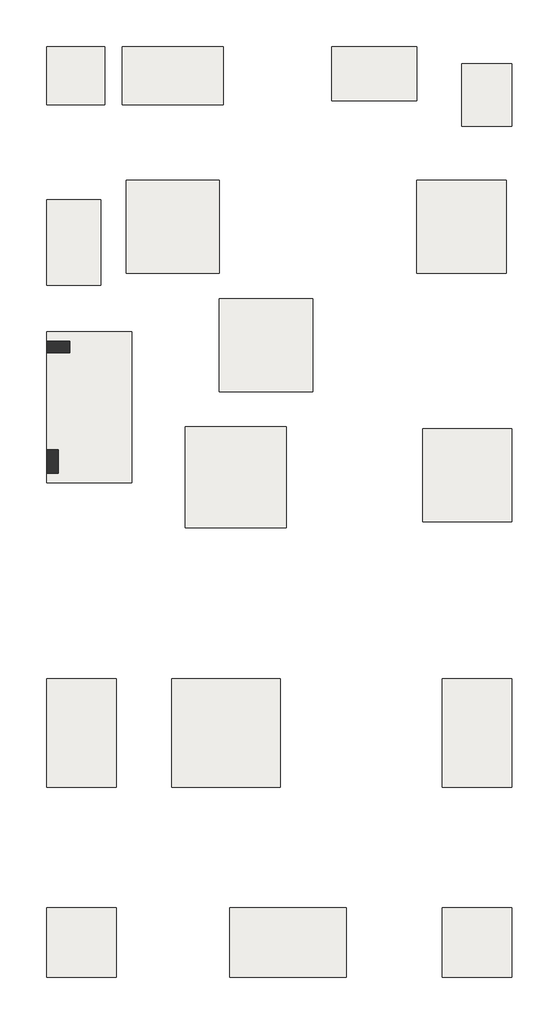
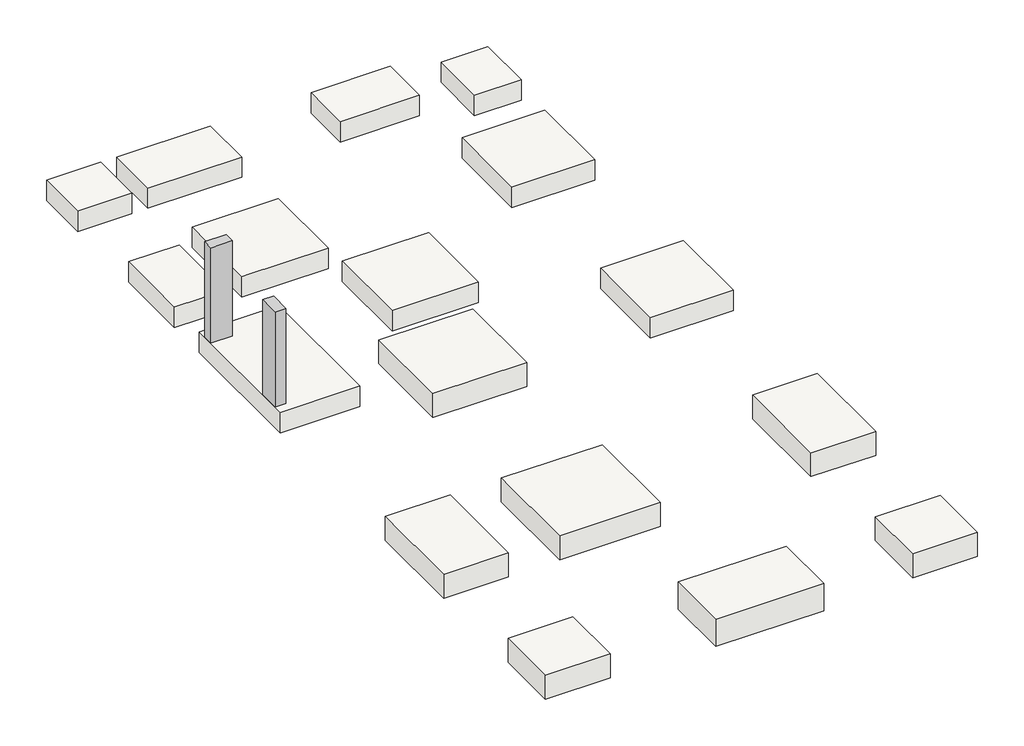
# One storey: 17 slabs, 2 columns.
"""IFC4 building model written with IfcOpenShell, lengths in millimetres."""

from ifc_helpers import new_model, si_unit, frame, origin, place, context, project, spatial, polyline, outline, extrude, transform, mapped, element, save
from components import slab_90c2f4b8, m_footing_rectangular_cf1_e8ad81a8, m_footing_rectangular_f1_8f1f0fab, m_footing_rectangular_f2_e38db0b8, m_footing_rectangular_f3_6d6a3403, m_footing_rectangular_f4_fcff0cd7, m_footing_rectangular_lp1_02c7f121, m_footing_rectangular_sf1_7ce3103a, m_footing_rectangular_sf2_5cd490c0, m_footing_rectangular_sf_4_edbcb53e, m_footing_rectangular_sf_5_e6d23758, m_footing_rectangular_sf3_0b37110f

model = new_model("IFC4")

# Units and contexts
model_context = context("Model", 3, world=origin())
ifc_project = project(units=[si_unit("LENGTHUNIT", "METRE", prefix="MILLI")], contexts=[model_context])

# Site, building, storey
site = spatial("IfcSite", under=ifc_project)
building = spatial("IfcBuilding", under=site)
storey = spatial("IfcBuildingStorey", under=building, Elevation=-2133.6)

# Columns
placement = place(None, origin())
element("IfcColumn", 1, ObjectType="M_Concrete-Rectangular-Column : 9\" x 18\"", at=placement, inside=storey, context=model_context, shape_type="SweptSolid", body=[
    extrude(outline(polyline([(18112.186814, 16783.9317951), (18112.186814, 16555.3317951), (17654.986814, 16555.3317951), (17654.986814, 16783.9317951), (18112.186814, 16783.9317951)])), frame((0.0, 0.0, -2133.6), z_axis=(0.0, 0.0, 1.0), x_axis=(1.0, 0.0, 0.0)), (0.0, 0.0, 1.0), 2133.6),
])
element("IfcColumn", 2, ObjectType="M_Concrete-Rectangular-Column : 9\" x 18\"", at=placement, inside=storey, context=model_context, shape_type="SweptSolid", body=[
    extrude(outline(polyline([(17654.986814, 14650.3317951), (17883.586814, 14650.3317951), (17883.586814, 14193.1317951), (17654.986814, 14193.1317951), (17654.986814, 14650.3317951)])), frame((0.0, 0.0, -2133.6), z_axis=(0.0, 0.0, 1.0), x_axis=(1.0, 0.0, 0.0)), (0.0, 0.0, 1.0), 2133.6),
])

# Slabs
slab_shape = slab_90c2f4b8(model_context)
element("IfcSlab", 3, ObjectType="M_Footing-Rectangular : 3'9\" x 3'9\"", at=placement, inside=storey, context=model_context, shape_type="MappedRepresentation", body=[
    mapped(slab_shape, transform((18226.486814, 22003.6317951, -2133.6), x_axis=(1.0, 0.0, 0.0), y_axis=(0.0, 1.0, 0.0), z_axis=(0.0, 0.0, 1.0))),
])
m_footing_rectangular_cf1_shape = m_footing_rectangular_cf1_e8ad81a8(model_context)
element("IfcSlab", 4, ObjectType="M_Footing-Rectangular : CF1", at=placement, inside=storey, context=model_context, shape_type="MappedRepresentation", body=[
    mapped(m_footing_rectangular_cf1_shape, transform((18340.786814, 4972.9317951, -2133.6), x_axis=(1.0, 0.0, 0.0), y_axis=(0.0, 1.0, 0.0), z_axis=(0.0, 0.0, 1.0))),
])
element("IfcSlab", 5, ObjectType="M_Footing-Rectangular : CF1", at=placement, inside=storey, context=model_context, shape_type="MappedRepresentation", body=[
    mapped(m_footing_rectangular_cf1_shape, transform((26113.186814, 4972.9317951, -2133.6), x_axis=(1.0, 0.0, 0.0), y_axis=(0.0, 1.0, 0.0), z_axis=(0.0, 0.0, 1.0))),
])
m_footing_rectangular_f1_shape = m_footing_rectangular_f1_8f1f0fab(model_context)
element("IfcSlab", 6, ObjectType="M_Footing-Rectangular : F1", at=placement, inside=storey, context=model_context, shape_type="MappedRepresentation", body=[
    mapped(m_footing_rectangular_f1_shape, transform((21178.6441916, 9087.7317951, -2133.6), x_axis=(1.0, 0.0, 0.0), y_axis=(0.0, 1.0, 0.0), z_axis=(0.0, 0.0, 1.0))),
])
m_footing_rectangular_f2_shape = m_footing_rectangular_f2_e38db0b8(model_context)
element("IfcSlab", 7, ObjectType="M_Footing-Rectangular : F2", at=placement, inside=storey, context=model_context, shape_type="MappedRepresentation", body=[
    mapped(m_footing_rectangular_f2_shape, transform((21369.1441916, 14116.9317951, -2133.6), x_axis=(1.0, 0.0, 0.0), y_axis=(0.0, 1.0, 0.0), z_axis=(0.0, 0.0, 1.0))),
])
m_footing_rectangular_f3_shape = m_footing_rectangular_f3_6d6a3403(model_context)
element("IfcSlab", 8, ObjectType="M_Footing-Rectangular : F3", at=placement, inside=storey, context=model_context, shape_type="MappedRepresentation", body=[
    mapped(m_footing_rectangular_f3_shape, transform((20131.486814, 19031.8317951, -2133.6), x_axis=(1.0, 0.0, 0.0), y_axis=(0.0, 1.0, 0.0), z_axis=(0.0, 0.0, 1.0))),
])
element("IfcSlab", 9, ObjectType="M_Footing-Rectangular : F3", at=placement, inside=storey, context=model_context, shape_type="MappedRepresentation", body=[
    mapped(m_footing_rectangular_f3_shape, transform((21966.0441916, 16707.7317951, -2133.6), x_axis=(1.0, 0.0, 0.0), y_axis=(0.0, 1.0, 0.0), z_axis=(0.0, 0.0, 1.0))),
])
m_footing_rectangular_f4_shape = m_footing_rectangular_f4_fcff0cd7(model_context)
element("IfcSlab", 10, ObjectType="M_Footing-Rectangular : F4", at=placement, inside=storey, context=model_context, shape_type="MappedRepresentation", body=[
    mapped(m_footing_rectangular_f4_shape, transform((25808.386814, 19031.8317951, -2133.6), x_axis=(1.0, 0.0, 0.0), y_axis=(0.0, 1.0, 0.0), z_axis=(0.0, 0.0, 1.0))),
])
element("IfcSlab", 11, ObjectType="M_Footing-Rectangular : F4", at=placement, inside=storey, context=model_context, shape_type="MappedRepresentation", body=[
    mapped(m_footing_rectangular_f4_shape, transform((25922.686814, 14155.0317951, -2133.6), x_axis=(1.0, 0.0, 0.0), y_axis=(0.0, 1.0, 0.0), z_axis=(0.0, 0.0, 1.0))),
])
m_footing_rectangular_lp1_shape = m_footing_rectangular_lp1_02c7f121(model_context)
element("IfcSlab", 12, ObjectType="M_Footing-Rectangular : LP1", at=placement, inside=storey, context=model_context, shape_type="MappedRepresentation", body=[
    mapped(m_footing_rectangular_lp1_shape, transform((18493.186814, 15488.5317951, -2133.6), x_axis=(0.0, 1.0, 0.0), y_axis=(-1.0, 0.0, 0.0), z_axis=(0.0, 0.0, 1.0))),
])
m_footing_rectangular_sf1_shape = m_footing_rectangular_sf1_7ce3103a(model_context)
element("IfcSlab", 13, ObjectType="M_Footing-Rectangular : SF1", at=placement, inside=storey, context=model_context, shape_type="MappedRepresentation", body=[
    mapped(m_footing_rectangular_sf1_shape, transform((22398.436814, 4972.9317951, -2133.6), x_axis=(0.0, 1.0, 0.0), y_axis=(-1.0, 0.0, 0.0), z_axis=(0.0, 0.0, 1.0))),
])
m_footing_rectangular_sf2_shape = m_footing_rectangular_sf2_5cd490c0(model_context)
element("IfcSlab", 14, ObjectType="M_Footing-Rectangular : SF2", at=placement, inside=storey, context=model_context, shape_type="MappedRepresentation", body=[
    mapped(m_footing_rectangular_sf2_shape, transform((26113.186814, 9087.7317951, -2133.6), x_axis=(1.0, 0.0, 0.0), y_axis=(0.0, 1.0, 0.0), z_axis=(0.0, 0.0, 1.0))),
])
element("IfcSlab", 15, ObjectType="M_Footing-Rectangular : SF2", at=placement, inside=storey, context=model_context, shape_type="MappedRepresentation", body=[
    mapped(m_footing_rectangular_sf2_shape, transform((18340.786814, 9087.7317951, -2133.6), x_axis=(1.0, 0.0, 0.0), y_axis=(0.0, 1.0, 0.0), z_axis=(0.0, 0.0, 1.0))),
])
m_footing_rectangular_sf_4_shape = m_footing_rectangular_sf_4_edbcb53e(model_context)
element("IfcSlab", 16, ObjectType="M_Footing-Rectangular : sf 4", at=placement, inside=storey, context=model_context, shape_type="MappedRepresentation", body=[
    mapped(m_footing_rectangular_sf_4_shape, transform((24093.4020345, 22041.7317951, -2133.6), x_axis=(1.0, 0.0, 0.0), y_axis=(0.0, 1.0, 0.0), z_axis=(0.0, 0.0, 1.0))),
])
element("IfcSlab", 17, ObjectType="M_Footing-Rectangular : sf 4", at=placement, inside=storey, context=model_context, shape_type="MappedRepresentation", body=[
    mapped(m_footing_rectangular_sf_4_shape, transform((18188.386814, 18727.0317951, -2133.6), x_axis=(0.0, 1.0, 0.0), y_axis=(-1.0, 0.0, 0.0), z_axis=(0.0, 0.0, 1.0))),
])
m_footing_rectangular_sf_5_shape = m_footing_rectangular_sf_5_e6d23758(model_context)
element("IfcSlab", 18, ObjectType="M_Footing-Rectangular : sf 5", at=placement, inside=storey, context=model_context, shape_type="MappedRepresentation", body=[
    mapped(m_footing_rectangular_sf_5_shape, transform((26303.686814, 21622.6317951, -2133.6), x_axis=(0.0, 1.0, 0.0), y_axis=(-1.0, 0.0, 0.0), z_axis=(0.0, 0.0, 1.0))),
])
m_footing_rectangular_sf3_shape = m_footing_rectangular_sf3_0b37110f(model_context)
element("IfcSlab", 19, ObjectType="M_Footing-Rectangular : sf3", at=placement, inside=storey, context=model_context, shape_type="MappedRepresentation", body=[
    mapped(m_footing_rectangular_sf3_shape, transform((20131.486814, 22003.6317951, -2133.6), x_axis=(1.0, 0.0, 0.0), y_axis=(0.0, 1.0, 0.0), z_axis=(0.0, 0.0, 1.0))),
])

save(model, "model.ifc")

# Revit data of these elements
# Type "M_Concrete-Rectangular-Column : 9\" x 18\""
#   b = 457.2 mm
#   h = 228.6 mm
#   Structural Material [instance default] = Concrete, Cast-in-Place gray
# Type "M_Footing-Rectangular : 3'9\" x 3'9\""
#   Width = 1143 mm
#   Length = 1143 mm
#   Foundation Thickness = 457.2 mm
#   Structural Material [instance default] = Concrete, Cast-in-Place gray
#   Assembly Code = ""
# Type "M_Footing-Rectangular : CF1"
#   Width = 1371.6 mm
#   Length = 1371.6 mm
#   Foundation Thickness = 533.4 mm
#   Structural Material [instance default] = Concrete, Cast-in-Place gray
#   Assembly Code = ""
# Type "M_Footing-Rectangular : F1"
#   Width = 2133.6 mm
#   Length = 2133.6 mm
#   Foundation Thickness = 533.4 mm
#   Structural Material [instance default] = Concrete, Cast-in-Place gray
#   Assembly Code = ""
# Type "M_Footing-Rectangular : F2"
#   Width = 1981.2 mm
#   Length = 1981.2 mm
#   Foundation Thickness = 533.4 mm
#   Structural Material [instance default] = Concrete, Cast-in-Place gray
#   Assembly Code = ""
# Type "M_Footing-Rectangular : F3"
#   Width = 1828.8 mm
#   Length = 1828.8 mm
#   Foundation Thickness = 457.2 mm
#   Structural Material [instance default] = Concrete, Cast-in-Place gray
#   Assembly Code = ""
# Type "M_Footing-Rectangular : F4"
#   Width = 1752.6 mm
#   Length = 1828.8 mm
#   Foundation Thickness = 457.2 mm
#   Structural Material [instance default] = Concrete, Cast-in-Place gray
#   Assembly Code = ""
# Type "M_Footing-Rectangular : LP1"
#   Width = 2971.8 mm
#   Length = 1676.4 mm
#   Foundation Thickness = 457.2 mm
#   Structural Material [instance default] = Concrete, Cast-in-Place gray
#   Assembly Code = ""
# Type "M_Footing-Rectangular : SF1"
#   Width = 1371.6 mm
#   Length = 2286 mm
#   Foundation Thickness = 609.6 mm
#   Structural Material [instance default] = Concrete, Cast-in-Place gray
#   Assembly Code = ""
# Type "M_Footing-Rectangular : SF2"
#   Width = 1371.6 mm
#   Length = 2133.6 mm
#   Foundation Thickness = 533.4 mm
#   Structural Material [instance default] = Concrete, Cast-in-Place gray
#   Assembly Code = ""
# Type "M_Footing-Rectangular : sf 4"
#   Width = 1676.4 mm
#   Length = 1066.8 mm
#   Foundation Thickness = 457.2 mm
#   Structural Material [instance default] = Concrete, Cast-in-Place gray
#   Assembly Code = ""
# Type "M_Footing-Rectangular : sf 5"
#   Width = 1219.2 mm
#   Length = 990.6 mm
#   Foundation Thickness = 457.2 mm
#   Structural Material [instance default] = Concrete, Cast-in-Place gray
#   Assembly Code = ""
# Type "M_Footing-Rectangular : sf3"
#   Width = 1981.2 mm
#   Length = 1143 mm
#   Foundation Thickness = 457.2 mm
#   Structural Material [instance default] = Concrete, Cast-in-Place gray
#   Assembly Code = ""
# Elements 1, 2 (IfcColumn, "M_Concrete-Rectangular-Column : 9\" x 18\"")
#   Structural Material = Concrete, Cast-in-Place gray
#   Phase Created = New Construction
#   Materials on its faces: "Concrete, Cast-in-Place gray"
# Element 3 (IfcSlab, "M_Footing-Rectangular : 3'9\" x 3'9\"")
#   Structural Material = Concrete, Cast-in-Place gray
#   Phase Created = New Construction
#   Materials on its faces: "Concrete, Cast-in-Place gray"
# Elements 4, 5 (IfcSlab, "M_Footing-Rectangular : CF1")
#   Structural Material = Concrete, Cast-in-Place gray
#   Phase Created = New Construction
#   Materials on its faces: "Concrete, Cast-in-Place gray"
# Element 6 (IfcSlab, "M_Footing-Rectangular : F1")
#   Structural Material = Concrete, Cast-in-Place gray
#   Phase Created = New Construction
#   Materials on its faces: "Concrete, Cast-in-Place gray"
# Element 7 (IfcSlab, "M_Footing-Rectangular : F2")
#   Structural Material = Concrete, Cast-in-Place gray
#   Phase Created = New Construction
#   Materials on its faces: "Concrete, Cast-in-Place gray"
# Elements 8, 9 (IfcSlab, "M_Footing-Rectangular : F3")
#   Structural Material = Concrete, Cast-in-Place gray
#   Phase Created = New Construction
#   Materials on its faces: "Concrete, Cast-in-Place gray"
# Elements 10, 11 (IfcSlab, "M_Footing-Rectangular : F4")
#   Structural Material = Concrete, Cast-in-Place gray
#   Phase Created = New Construction
#   Materials on its faces: "Concrete, Cast-in-Place gray"
# Element 12 (IfcSlab, "M_Footing-Rectangular : LP1")
#   Structural Material = Concrete, Cast-in-Place gray
#   Phase Created = New Construction
#   Materials on its faces: "Concrete, Cast-in-Place gray"
# Element 13 (IfcSlab, "M_Footing-Rectangular : SF1")
#   Structural Material = Concrete, Cast-in-Place gray
#   Phase Created = New Construction
#   Materials on its faces: "Concrete, Cast-in-Place gray"
# Elements 14, 15 (IfcSlab, "M_Footing-Rectangular : SF2")
#   Structural Material = Concrete, Cast-in-Place gray
#   Phase Created = New Construction
#   Materials on its faces: "Concrete, Cast-in-Place gray"
# Elements 16, 17 (IfcSlab, "M_Footing-Rectangular : sf 4")
#   Structural Material = Concrete, Cast-in-Place gray
#   Phase Created = New Construction
#   Materials on its faces: "Concrete, Cast-in-Place gray"
# Element 18 (IfcSlab, "M_Footing-Rectangular : sf 5")
#   Structural Material = Concrete, Cast-in-Place gray
#   Phase Created = New Construction
#   Materials on its faces: "Concrete, Cast-in-Place gray"
# Element 19 (IfcSlab, "M_Footing-Rectangular : sf3")
#   Structural Material = Concrete, Cast-in-Place gray
#   Phase Created = New Construction
#   Materials on its faces: "Concrete, Cast-in-Place gray"
# Materials
#   "Concrete, Cast-in-Place gray": class "Concrete", colour RGB 192 192 192, transparency 0, Description = "Cast-in-place concrete", Cost = 0
